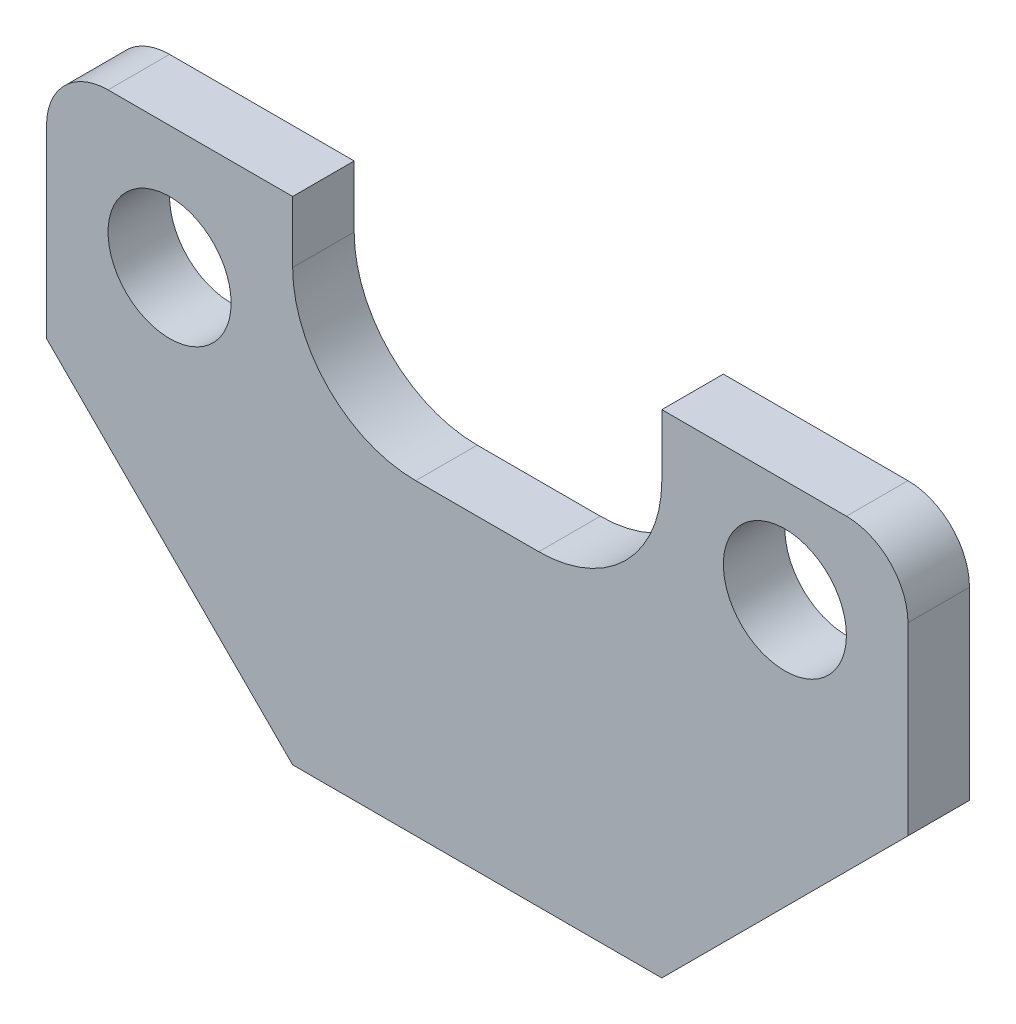
ISO-10303-21;
HEADER;
FILE_DESCRIPTION(('STEP AP214'),'2;1');
FILE_NAME('part.step','',(''),(''),'','','');
FILE_SCHEMA(('AUTOMOTIVE_DESIGN { 1 0 10303 214 1 1 1 1 }'));
ENDSEC;
DATA;
#1=APPLICATION_CONTEXT('core data for automotive mechanical design processes');
#2=APPLICATION_PROTOCOL_DEFINITION('international standard','automotive_design',2000,#1);
#3=PRODUCT_CONTEXT('',#1,'mechanical');
#4=PRODUCT('Part','Part','',(#3));
#5=PRODUCT_RELATED_PRODUCT_CATEGORY('part','',(#4));
#6=PRODUCT_DEFINITION_FORMATION('','',#4);
#7=PRODUCT_DEFINITION_CONTEXT('part definition',#1,'design');
#8=PRODUCT_DEFINITION('design','',#6,#7);
#9=PRODUCT_DEFINITION_SHAPE('','',#8);
#10=(LENGTH_UNIT() NAMED_UNIT(*) SI_UNIT(.MILLI.,.METRE.));
#11=(NAMED_UNIT(*) PLANE_ANGLE_UNIT() SI_UNIT($,.RADIAN.));
#12=(NAMED_UNIT(*) SI_UNIT($,.STERADIAN.) SOLID_ANGLE_UNIT());
#13=UNCERTAINTY_MEASURE_WITH_UNIT(LENGTH_MEASURE(1.E-05),#10,'distance_accuracy_value','');
#14=(GEOMETRIC_REPRESENTATION_CONTEXT(3) GLOBAL_UNCERTAINTY_ASSIGNED_CONTEXT((#13)) GLOBAL_UNIT_ASSIGNED_CONTEXT((#10,
#11,#12)) REPRESENTATION_CONTEXT('',''));
#15=CARTESIAN_POINT('',(0.,0.,0.));
#16=DIRECTION('',(0.,0.,1.));
#17=DIRECTION('',(1.,0.,0.));
#18=AXIS2_PLACEMENT_3D('',#15,#16,#17);
#19=CARTESIAN_POINT('',(0.,0.,5.));
#20=DIRECTION('',(0.707106781186548,0.707106781186548,0.));
#21=DIRECTION('',(-0.707106781186548,0.707106781186548,0.));
#22=AXIS2_PLACEMENT_3D('',#19,#20,#21);
#23=PLANE('',#22);
#24=DIRECTION('',(0.707106781186548,-0.707106781186548,0.));
#25=VECTOR('',#24,1.);
#26=CARTESIAN_POINT('',(0.,0.,0.));
#27=LINE('',#26,#25);
#28=CARTESIAN_POINT('',(-20.,20.,0.));
#29=VERTEX_POINT('',#28);
#30=CARTESIAN_POINT('',(0.,0.,0.));
#31=VERTEX_POINT('',#30);
#32=EDGE_CURVE('E169',#29,#31,#27,.T.);
#33=ORIENTED_EDGE('',*,*,#32,.T.);
#34=DIRECTION('',(0.,0.,-1.));
#35=VECTOR('',#34,1.);
#36=CARTESIAN_POINT('',(0.,0.,5.));
#37=LINE('',#36,#35);
#38=CARTESIAN_POINT('',(0.,0.,5.));
#39=VERTEX_POINT('',#38);
#40=EDGE_CURVE('E147',#39,#31,#37,.T.);
#41=ORIENTED_EDGE('',*,*,#40,.F.);
#42=DIRECTION('',(0.707106781186548,-0.707106781186548,0.));
#43=VECTOR('',#42,1.);
#44=CARTESIAN_POINT('',(0.,0.,5.));
#45=LINE('',#44,#43);
#46=CARTESIAN_POINT('',(-20.,20.,5.));
#47=VERTEX_POINT('',#46);
#48=EDGE_CURVE('E156',#47,#39,#45,.T.);
#49=ORIENTED_EDGE('',*,*,#48,.F.);
#50=DIRECTION('',(0.,0.,-1.));
#51=VECTOR('',#50,1.);
#52=CARTESIAN_POINT('',(-20.,20.,5.));
#53=LINE('',#52,#51);
#54=EDGE_CURVE('E203',#47,#29,#53,.T.);
#55=ORIENTED_EDGE('',*,*,#54,.T.);
#56=EDGE_LOOP('',(#33,#41,#49,#55));
#57=FACE_BOUND('',#56,.T.);
#58=ADVANCED_FACE('F44',(#57),#23,.F.);
#59=CARTESIAN_POINT('',(0.,0.,5.));
#60=DIRECTION('',(0.,1.,0.));
#61=DIRECTION('',(0.,0.,1.));
#62=AXIS2_PLACEMENT_3D('',#59,#60,#61);
#63=PLANE('',#62);
#64=DIRECTION('',(1.,0.,0.));
#65=VECTOR('',#64,1.);
#66=CARTESIAN_POINT('',(0.,0.,0.));
#67=LINE('',#66,#65);
#68=CARTESIAN_POINT('',(30.,0.,0.));
#69=VERTEX_POINT('',#68);
#70=EDGE_CURVE('E240',#31,#69,#67,.T.);
#71=ORIENTED_EDGE('',*,*,#70,.T.);
#72=DIRECTION('',(0.,0.,-1.));
#73=VECTOR('',#72,1.);
#74=CARTESIAN_POINT('',(30.,0.,5.));
#75=LINE('',#74,#73);
#76=CARTESIAN_POINT('',(30.,0.,5.));
#77=VERTEX_POINT('',#76);
#78=EDGE_CURVE('E153',#77,#69,#75,.T.);
#79=ORIENTED_EDGE('',*,*,#78,.F.);
#80=DIRECTION('',(1.,0.,0.));
#81=VECTOR('',#80,1.);
#82=CARTESIAN_POINT('',(0.,0.,5.));
#83=LINE('',#82,#81);
#84=EDGE_CURVE('E148',#39,#77,#83,.T.);
#85=ORIENTED_EDGE('',*,*,#84,.F.);
#86=ORIENTED_EDGE('',*,*,#40,.T.);
#87=EDGE_LOOP('',(#71,#79,#85,#86));
#88=FACE_BOUND('',#87,.T.);
#89=ADVANCED_FACE('F146',(#88),#63,.F.);
#90=CARTESIAN_POINT('',(30.,0.,5.));
#91=DIRECTION('',(-0.707106781186547,0.707106781186548,0.));
#92=DIRECTION('',(-0.707106781186548,-0.707106781186547,0.));
#93=AXIS2_PLACEMENT_3D('',#90,#91,#92);
#94=PLANE('',#93);
#95=DIRECTION('',(0.707106781186548,0.707106781186547,0.));
#96=VECTOR('',#95,1.);
#97=CARTESIAN_POINT('',(30.,0.,0.));
#98=LINE('',#97,#96);
#99=CARTESIAN_POINT('',(50.,20.,0.));
#100=VERTEX_POINT('',#99);
#101=EDGE_CURVE('E234',#69,#100,#98,.T.);
#102=ORIENTED_EDGE('',*,*,#101,.T.);
#103=DIRECTION('',(0.,0.,-1.));
#104=VECTOR('',#103,1.);
#105=CARTESIAN_POINT('',(50.,20.,5.));
#106=LINE('',#105,#104);
#107=CARTESIAN_POINT('',(50.,20.,5.));
#108=VERTEX_POINT('',#107);
#109=EDGE_CURVE('E173',#108,#100,#106,.T.);
#110=ORIENTED_EDGE('',*,*,#109,.F.);
#111=DIRECTION('',(0.707106781186548,0.707106781186547,0.));
#112=VECTOR('',#111,1.);
#113=CARTESIAN_POINT('',(30.,0.,5.));
#114=LINE('',#113,#112);
#115=EDGE_CURVE('E154',#77,#108,#114,.T.);
#116=ORIENTED_EDGE('',*,*,#115,.F.);
#117=ORIENTED_EDGE('',*,*,#78,.T.);
#118=EDGE_LOOP('',(#102,#110,#116,#117));
#119=FACE_BOUND('',#118,.T.);
#120=ADVANCED_FACE('F262',(#119),#94,.F.);
#121=CARTESIAN_POINT('',(50.,40.,5.));
#122=DIRECTION('',(-1.,0.,0.));
#123=DIRECTION('',(0.,0.,1.));
#124=AXIS2_PLACEMENT_3D('',#121,#122,#123);
#125=PLANE('',#124);
#126=DIRECTION('',(0.,1.,0.));
#127=VECTOR('',#126,1.);
#128=CARTESIAN_POINT('',(50.,40.,0.));
#129=LINE('',#128,#127);
#130=CARTESIAN_POINT('',(50.,35.,0.));
#131=VERTEX_POINT('',#130);
#132=EDGE_CURVE('E227',#100,#131,#129,.T.);
#133=ORIENTED_EDGE('',*,*,#132,.T.);
#134=DIRECTION('',(0.,0.,-1.));
#135=VECTOR('',#134,1.);
#136=CARTESIAN_POINT('',(50.,35.,5.));
#137=LINE('',#136,#135);
#138=CARTESIAN_POINT('',(50.,35.,5.));
#139=VERTEX_POINT('',#138);
#140=EDGE_CURVE('E182',#131,#139,#137,.F.);
#141=ORIENTED_EDGE('',*,*,#140,.T.);
#142=DIRECTION('',(0.,1.,0.));
#143=VECTOR('',#142,1.);
#144=CARTESIAN_POINT('',(50.,40.,5.));
#145=LINE('',#144,#143);
#146=EDGE_CURVE('E228',#108,#139,#145,.T.);
#147=ORIENTED_EDGE('',*,*,#146,.F.);
#148=ORIENTED_EDGE('',*,*,#109,.T.);
#149=EDGE_LOOP('',(#133,#141,#147,#148));
#150=FACE_BOUND('',#149,.T.);
#151=ADVANCED_FACE('F226',(#150),#125,.F.);
#152=CARTESIAN_POINT('',(30.,40.,5.));
#153=DIRECTION('',(0.,-1.,0.));
#154=DIRECTION('',(0.,0.,-1.));
#155=AXIS2_PLACEMENT_3D('',#152,#153,#154);
#156=PLANE('',#155);
#157=DIRECTION('',(-1.,0.,0.));
#158=VECTOR('',#157,1.);
#159=CARTESIAN_POINT('',(30.,40.,5.));
#160=LINE('',#159,#158);
#161=CARTESIAN_POINT('',(45.,40.,5.));
#162=VERTEX_POINT('',#161);
#163=CARTESIAN_POINT('',(30.,40.,5.));
#164=VERTEX_POINT('',#163);
#165=EDGE_CURVE('E266',#162,#164,#160,.T.);
#166=ORIENTED_EDGE('',*,*,#165,.F.);
#167=DIRECTION('',(0.,0.,-1.));
#168=VECTOR('',#167,1.);
#169=CARTESIAN_POINT('',(45.,40.,5.));
#170=LINE('',#169,#168);
#171=CARTESIAN_POINT('',(45.,40.,0.));
#172=VERTEX_POINT('',#171);
#173=EDGE_CURVE('E166',#162,#172,#170,.T.);
#174=ORIENTED_EDGE('',*,*,#173,.T.);
#175=DIRECTION('',(-1.,0.,0.));
#176=VECTOR('',#175,1.);
#177=CARTESIAN_POINT('',(30.,40.,0.));
#178=LINE('',#177,#176);
#179=CARTESIAN_POINT('',(30.,40.,0.));
#180=VERTEX_POINT('',#179);
#181=EDGE_CURVE('E232',#172,#180,#178,.T.);
#182=ORIENTED_EDGE('',*,*,#181,.T.);
#183=DIRECTION('',(0.,0.,-1.));
#184=VECTOR('',#183,1.);
#185=CARTESIAN_POINT('',(30.,40.,5.));
#186=LINE('',#185,#184);
#187=EDGE_CURVE('E217',#164,#180,#186,.T.);
#188=ORIENTED_EDGE('',*,*,#187,.F.);
#189=EDGE_LOOP('',(#166,#174,#182,#188));
#190=FACE_BOUND('',#189,.T.);
#191=ADVANCED_FACE('F296',(#190),#156,.F.);
#192=CARTESIAN_POINT('',(30.,35.,5.));
#193=DIRECTION('',(1.,0.,0.));
#194=DIRECTION('',(0.,0.,-1.));
#195=AXIS2_PLACEMENT_3D('',#192,#193,#194);
#196=PLANE('',#195);
#197=DIRECTION('',(0.,-1.,0.));
#198=VECTOR('',#197,1.);
#199=CARTESIAN_POINT('',(30.,35.,0.));
#200=LINE('',#199,#198);
#201=CARTESIAN_POINT('',(30.,35.,0.));
#202=VERTEX_POINT('',#201);
#203=EDGE_CURVE('E231',#180,#202,#200,.T.);
#204=ORIENTED_EDGE('',*,*,#203,.T.);
#205=DIRECTION('',(0.,0.,-1.));
#206=VECTOR('',#205,1.);
#207=CARTESIAN_POINT('',(30.,35.,5.));
#208=LINE('',#207,#206);
#209=CARTESIAN_POINT('',(30.,35.,5.));
#210=VERTEX_POINT('',#209);
#211=EDGE_CURVE('E214',#210,#202,#208,.T.);
#212=ORIENTED_EDGE('',*,*,#211,.F.);
#213=DIRECTION('',(0.,-1.,0.));
#214=VECTOR('',#213,1.);
#215=CARTESIAN_POINT('',(30.,35.,5.));
#216=LINE('',#215,#214);
#217=EDGE_CURVE('E269',#164,#210,#216,.T.);
#218=ORIENTED_EDGE('',*,*,#217,.F.);
#219=ORIENTED_EDGE('',*,*,#187,.T.);
#220=EDGE_LOOP('',(#204,#212,#218,#219));
#221=FACE_BOUND('',#220,.T.);
#222=ADVANCED_FACE('F295',(#221),#196,.F.);
#223=CARTESIAN_POINT('',(20.,35.,5.));
#224=DIRECTION('',(0.,0.,-1.));
#225=DIRECTION('',(-1.,0.,0.));
#226=AXIS2_PLACEMENT_3D('',#223,#224,#225);
#227=CYLINDRICAL_SURFACE('',#226,10.);
#228=CARTESIAN_POINT('',(20.,35.,0.));
#229=DIRECTION('',(0.,0.,-1.));
#230=DIRECTION('',(1.,0.,0.));
#231=AXIS2_PLACEMENT_3D('',#228,#229,#230);
#232=CIRCLE('',#231,10.);
#233=CARTESIAN_POINT('',(20.,25.,0.));
#234=VERTEX_POINT('',#233);
#235=EDGE_CURVE('E242',#202,#234,#232,.T.);
#236=ORIENTED_EDGE('',*,*,#235,.T.);
#237=DIRECTION('',(0.,0.,-1.));
#238=VECTOR('',#237,1.);
#239=CARTESIAN_POINT('',(20.,25.,5.));
#240=LINE('',#239,#238);
#241=CARTESIAN_POINT('',(20.,25.,5.));
#242=VERTEX_POINT('',#241);
#243=EDGE_CURVE('E215',#242,#234,#240,.T.);
#244=ORIENTED_EDGE('',*,*,#243,.F.);
#245=CARTESIAN_POINT('',(20.,35.,5.));
#246=DIRECTION('',(0.,0.,-1.));
#247=DIRECTION('',(1.,0.,0.));
#248=AXIS2_PLACEMENT_3D('',#245,#246,#247);
#249=CIRCLE('',#248,10.);
#250=EDGE_CURVE('E275',#210,#242,#249,.T.);
#251=ORIENTED_EDGE('',*,*,#250,.F.);
#252=ORIENTED_EDGE('',*,*,#211,.T.);
#253=EDGE_LOOP('',(#236,#244,#251,#252));
#254=FACE_BOUND('',#253,.T.);
#255=ADVANCED_FACE('F287',(#254),#227,.F.);
#256=CARTESIAN_POINT('',(10.,25.,5.));
#257=DIRECTION('',(0.,-1.,0.));
#258=DIRECTION('',(0.,0.,-1.));
#259=AXIS2_PLACEMENT_3D('',#256,#257,#258);
#260=PLANE('',#259);
#261=DIRECTION('',(-1.,0.,0.));
#262=VECTOR('',#261,1.);
#263=CARTESIAN_POINT('',(10.,25.,0.));
#264=LINE('',#263,#262);
#265=CARTESIAN_POINT('',(10.,25.,0.));
#266=VERTEX_POINT('',#265);
#267=EDGE_CURVE('E243',#234,#266,#264,.T.);
#268=ORIENTED_EDGE('',*,*,#267,.T.);
#269=DIRECTION('',(0.,0.,-1.));
#270=VECTOR('',#269,1.);
#271=CARTESIAN_POINT('',(10.,25.,5.));
#272=LINE('',#271,#270);
#273=CARTESIAN_POINT('',(10.,25.,5.));
#274=VERTEX_POINT('',#273);
#275=EDGE_CURVE('E207',#274,#266,#272,.T.);
#276=ORIENTED_EDGE('',*,*,#275,.F.);
#277=DIRECTION('',(-1.,0.,0.));
#278=VECTOR('',#277,1.);
#279=CARTESIAN_POINT('',(10.,25.,5.));
#280=LINE('',#279,#278);
#281=EDGE_CURVE('E273',#242,#274,#280,.T.);
#282=ORIENTED_EDGE('',*,*,#281,.F.);
#283=ORIENTED_EDGE('',*,*,#243,.T.);
#284=EDGE_LOOP('',(#268,#276,#282,#283));
#285=FACE_BOUND('',#284,.T.);
#286=ADVANCED_FACE('F283',(#285),#260,.F.);
#287=CARTESIAN_POINT('',(10.,35.,5.));
#288=DIRECTION('',(0.,0.,-1.));
#289=DIRECTION('',(-1.,0.,0.));
#290=AXIS2_PLACEMENT_3D('',#287,#288,#289);
#291=CYLINDRICAL_SURFACE('',#290,10.);
#292=CARTESIAN_POINT('',(10.,35.,0.));
#293=DIRECTION('',(0.,0.,-1.));
#294=DIRECTION('',(1.,0.,0.));
#295=AXIS2_PLACEMENT_3D('',#292,#293,#294);
#296=CIRCLE('',#295,10.);
#297=CARTESIAN_POINT('',(0.,35.,0.));
#298=VERTEX_POINT('',#297);
#299=EDGE_CURVE('E248',#266,#298,#296,.T.);
#300=ORIENTED_EDGE('',*,*,#299,.T.);
#301=DIRECTION('',(0.,0.,-1.));
#302=VECTOR('',#301,1.);
#303=CARTESIAN_POINT('',(0.,35.,5.));
#304=LINE('',#303,#302);
#305=CARTESIAN_POINT('',(0.,35.,5.));
#306=VERTEX_POINT('',#305);
#307=EDGE_CURVE('E206',#306,#298,#304,.T.);
#308=ORIENTED_EDGE('',*,*,#307,.F.);
#309=CARTESIAN_POINT('',(10.,35.,5.));
#310=DIRECTION('',(0.,0.,-1.));
#311=DIRECTION('',(1.,0.,0.));
#312=AXIS2_PLACEMENT_3D('',#309,#310,#311);
#313=CIRCLE('',#312,10.);
#314=EDGE_CURVE('E259',#274,#306,#313,.T.);
#315=ORIENTED_EDGE('',*,*,#314,.F.);
#316=ORIENTED_EDGE('',*,*,#275,.T.);
#317=EDGE_LOOP('',(#300,#308,#315,#316));
#318=FACE_BOUND('',#317,.T.);
#319=ADVANCED_FACE('F276',(#318),#291,.F.);
#320=CARTESIAN_POINT('',(0.,40.,5.));
#321=DIRECTION('',(-1.,0.,0.));
#322=DIRECTION('',(0.,0.,1.));
#323=AXIS2_PLACEMENT_3D('',#320,#321,#322);
#324=PLANE('',#323);
#325=DIRECTION('',(0.,1.,0.));
#326=VECTOR('',#325,1.);
#327=CARTESIAN_POINT('',(0.,40.,0.));
#328=LINE('',#327,#326);
#329=CARTESIAN_POINT('',(0.,40.,0.));
#330=VERTEX_POINT('',#329);
#331=EDGE_CURVE('E197',#298,#330,#328,.T.);
#332=ORIENTED_EDGE('',*,*,#331,.T.);
#333=DIRECTION('',(0.,0.,-1.));
#334=VECTOR('',#333,1.);
#335=CARTESIAN_POINT('',(0.,40.,5.));
#336=LINE('',#335,#334);
#337=CARTESIAN_POINT('',(0.,40.,5.));
#338=VERTEX_POINT('',#337);
#339=EDGE_CURVE('E201',#338,#330,#336,.T.);
#340=ORIENTED_EDGE('',*,*,#339,.F.);
#341=DIRECTION('',(0.,1.,0.));
#342=VECTOR('',#341,1.);
#343=CARTESIAN_POINT('',(0.,40.,5.));
#344=LINE('',#343,#342);
#345=EDGE_CURVE('E258',#306,#338,#344,.T.);
#346=ORIENTED_EDGE('',*,*,#345,.F.);
#347=ORIENTED_EDGE('',*,*,#307,.T.);
#348=EDGE_LOOP('',(#332,#340,#346,#347));
#349=FACE_BOUND('',#348,.T.);
#350=ADVANCED_FACE('F246',(#349),#324,.F.);
#351=CARTESIAN_POINT('',(0.,40.,5.));
#352=DIRECTION('',(0.,-1.,0.));
#353=DIRECTION('',(0.,0.,-1.));
#354=AXIS2_PLACEMENT_3D('',#351,#352,#353);
#355=PLANE('',#354);
#356=DIRECTION('',(-1.,0.,0.));
#357=VECTOR('',#356,1.);
#358=CARTESIAN_POINT('',(0.,40.,0.));
#359=LINE('',#358,#357);
#360=CARTESIAN_POINT('',(-15.,40.,0.));
#361=VERTEX_POINT('',#360);
#362=EDGE_CURVE('E191',#330,#361,#359,.T.);
#363=ORIENTED_EDGE('',*,*,#362,.T.);
#364=DIRECTION('',(0.,0.,-1.));
#365=VECTOR('',#364,1.);
#366=CARTESIAN_POINT('',(-15.,40.,5.));
#367=LINE('',#366,#365);
#368=CARTESIAN_POINT('',(-15.,40.,5.));
#369=VERTEX_POINT('',#368);
#370=EDGE_CURVE('E11',#361,#369,#367,.F.);
#371=ORIENTED_EDGE('',*,*,#370,.T.);
#372=DIRECTION('',(-1.,0.,0.));
#373=VECTOR('',#372,1.);
#374=CARTESIAN_POINT('',(0.,40.,5.));
#375=LINE('',#374,#373);
#376=EDGE_CURVE('E254',#338,#369,#375,.T.);
#377=ORIENTED_EDGE('',*,*,#376,.F.);
#378=ORIENTED_EDGE('',*,*,#339,.T.);
#379=EDGE_LOOP('',(#363,#371,#377,#378));
#380=FACE_BOUND('',#379,.T.);
#381=ADVANCED_FACE('F255',(#380),#355,.F.);
#382=CARTESIAN_POINT('',(-20.,40.,5.));
#383=DIRECTION('',(1.,0.,0.));
#384=DIRECTION('',(0.,0.,-1.));
#385=AXIS2_PLACEMENT_3D('',#382,#383,#384);
#386=PLANE('',#385);
#387=DIRECTION('',(0.,-1.,0.));
#388=VECTOR('',#387,1.);
#389=CARTESIAN_POINT('',(-20.,40.,5.));
#390=LINE('',#389,#388);
#391=CARTESIAN_POINT('',(-20.,35.,5.));
#392=VERTEX_POINT('',#391);
#393=EDGE_CURVE('E161',#392,#47,#390,.T.);
#394=ORIENTED_EDGE('',*,*,#393,.F.);
#395=DIRECTION('',(0.,0.,-1.));
#396=VECTOR('',#395,1.);
#397=CARTESIAN_POINT('',(-20.,35.,5.));
#398=LINE('',#397,#396);
#399=CARTESIAN_POINT('',(-20.,35.,0.));
#400=VERTEX_POINT('',#399);
#401=EDGE_CURVE('E52',#392,#400,#398,.T.);
#402=ORIENTED_EDGE('',*,*,#401,.T.);
#403=DIRECTION('',(0.,-1.,0.));
#404=VECTOR('',#403,1.);
#405=CARTESIAN_POINT('',(-20.,40.,0.));
#406=LINE('',#405,#404);
#407=EDGE_CURVE('E164',#400,#29,#406,.T.);
#408=ORIENTED_EDGE('',*,*,#407,.T.);
#409=ORIENTED_EDGE('',*,*,#54,.F.);
#410=EDGE_LOOP('',(#394,#402,#408,#409));
#411=FACE_BOUND('',#410,.T.);
#412=ADVANCED_FACE('F188',(#411),#386,.F.);
#413=CARTESIAN_POINT('',(10.,35.,5.));
#414=DIRECTION('',(0.,0.,1.));
#415=DIRECTION('',(1.,0.,0.));
#416=AXIS2_PLACEMENT_3D('',#413,#414,#415);
#417=PLANE('',#416);
#418=CARTESIAN_POINT('',(40.,31.6094695208061,5.));
#419=DIRECTION('',(0.,0.,1.));
#420=DIRECTION('',(1.,0.,0.));
#421=AXIS2_PLACEMENT_3D('',#418,#419,#420);
#422=CIRCLE('',#421,5.);
#423=CARTESIAN_POINT('',(45.,31.6094695208061,5.));
#424=VERTEX_POINT('',#423);
#425=EDGE_CURVE('E357',#424,#424,#422,.T.);
#426=ORIENTED_EDGE('',*,*,#425,.F.);
#427=EDGE_LOOP('',(#426));
#428=FACE_BOUND('',#427,.T.);
#429=CARTESIAN_POINT('',(-10.,30.,5.));
#430=DIRECTION('',(0.,0.,1.));
#431=DIRECTION('',(1.,0.,0.));
#432=AXIS2_PLACEMENT_3D('',#429,#430,#431);
#433=CIRCLE('',#432,5.);
#434=CARTESIAN_POINT('',(-5.,30.,5.));
#435=VERTEX_POINT('',#434);
#436=EDGE_CURVE('E352',#435,#435,#433,.T.);
#437=ORIENTED_EDGE('',*,*,#436,.F.);
#438=EDGE_LOOP('',(#437));
#439=FACE_BOUND('',#438,.T.);
#440=ORIENTED_EDGE('',*,*,#146,.T.);
#441=CARTESIAN_POINT('',(45.,35.,5.));
#442=DIRECTION('',(0.,0.,1.));
#443=DIRECTION('',(1.,0.,0.));
#444=AXIS2_PLACEMENT_3D('',#441,#442,#443);
#445=CIRCLE('',#444,5.);
#446=EDGE_CURVE('E184',#139,#162,#445,.T.);
#447=ORIENTED_EDGE('',*,*,#446,.T.);
#448=ORIENTED_EDGE('',*,*,#165,.T.);
#449=ORIENTED_EDGE('',*,*,#217,.T.);
#450=ORIENTED_EDGE('',*,*,#250,.T.);
#451=ORIENTED_EDGE('',*,*,#281,.T.);
#452=ORIENTED_EDGE('',*,*,#314,.T.);
#453=ORIENTED_EDGE('',*,*,#345,.T.);
#454=ORIENTED_EDGE('',*,*,#376,.T.);
#455=CARTESIAN_POINT('',(-15.,35.,5.));
#456=DIRECTION('',(0.,0.,1.));
#457=DIRECTION('',(1.,0.,0.));
#458=AXIS2_PLACEMENT_3D('',#455,#456,#457);
#459=CIRCLE('',#458,5.);
#460=EDGE_CURVE('E58',#369,#392,#459,.T.);
#461=ORIENTED_EDGE('',*,*,#460,.T.);
#462=ORIENTED_EDGE('',*,*,#393,.T.);
#463=ORIENTED_EDGE('',*,*,#48,.T.);
#464=ORIENTED_EDGE('',*,*,#84,.T.);
#465=ORIENTED_EDGE('',*,*,#115,.T.);
#466=EDGE_LOOP('',(#440,#447,#448,#449,#450,#451,#452,#453,#454,#461,#462,#463,#464,#465));
#467=FACE_BOUND('',#466,.T.);
#468=ADVANCED_FACE('F159',(#428,#439,#467),#417,.T.);
#469=CARTESIAN_POINT('',(10.,35.,0.));
#470=DIRECTION('',(0.,0.,1.));
#471=DIRECTION('',(1.,0.,0.));
#472=AXIS2_PLACEMENT_3D('',#469,#470,#471);
#473=PLANE('',#472);
#474=CARTESIAN_POINT('',(40.,31.6094695208061,0.));
#475=DIRECTION('',(0.,0.,1.));
#476=DIRECTION('',(1.,0.,0.));
#477=AXIS2_PLACEMENT_3D('',#474,#475,#476);
#478=CIRCLE('',#477,5.);
#479=CARTESIAN_POINT('',(45.,31.6094695208061,0.));
#480=VERTEX_POINT('',#479);
#481=EDGE_CURVE('E353',#480,#480,#478,.T.);
#482=ORIENTED_EDGE('',*,*,#481,.T.);
#483=EDGE_LOOP('',(#482));
#484=FACE_BOUND('',#483,.T.);
#485=CARTESIAN_POINT('',(-10.,30.,0.));
#486=DIRECTION('',(0.,0.,1.));
#487=DIRECTION('',(1.,0.,0.));
#488=AXIS2_PLACEMENT_3D('',#485,#486,#487);
#489=CIRCLE('',#488,5.);
#490=CARTESIAN_POINT('',(-5.,30.,0.));
#491=VERTEX_POINT('',#490);
#492=EDGE_CURVE('E263',#491,#491,#489,.T.);
#493=ORIENTED_EDGE('',*,*,#492,.T.);
#494=EDGE_LOOP('',(#493));
#495=FACE_BOUND('',#494,.T.);
#496=ORIENTED_EDGE('',*,*,#181,.F.);
#497=CARTESIAN_POINT('',(45.,35.,0.));
#498=DIRECTION('',(0.,0.,1.));
#499=DIRECTION('',(1.,0.,0.));
#500=AXIS2_PLACEMENT_3D('',#497,#498,#499);
#501=CIRCLE('',#500,5.);
#502=EDGE_CURVE('E180',#172,#131,#501,.F.);
#503=ORIENTED_EDGE('',*,*,#502,.T.);
#504=ORIENTED_EDGE('',*,*,#132,.F.);
#505=ORIENTED_EDGE('',*,*,#101,.F.);
#506=ORIENTED_EDGE('',*,*,#70,.F.);
#507=ORIENTED_EDGE('',*,*,#32,.F.);
#508=ORIENTED_EDGE('',*,*,#407,.F.);
#509=CARTESIAN_POINT('',(-15.,35.,0.));
#510=DIRECTION('',(0.,0.,1.));
#511=DIRECTION('',(1.,0.,0.));
#512=AXIS2_PLACEMENT_3D('',#509,#510,#511);
#513=CIRCLE('',#512,5.);
#514=EDGE_CURVE('E172',#400,#361,#513,.F.);
#515=ORIENTED_EDGE('',*,*,#514,.T.);
#516=ORIENTED_EDGE('',*,*,#362,.F.);
#517=ORIENTED_EDGE('',*,*,#331,.F.);
#518=ORIENTED_EDGE('',*,*,#299,.F.);
#519=ORIENTED_EDGE('',*,*,#267,.F.);
#520=ORIENTED_EDGE('',*,*,#235,.F.);
#521=ORIENTED_EDGE('',*,*,#203,.F.);
#522=EDGE_LOOP('',(#496,#503,#504,#505,#506,#507,#508,#515,#516,#517,#518,#519,#520,#521));
#523=FACE_BOUND('',#522,.T.);
#524=ADVANCED_FACE('F192',(#484,#495,#523),#473,.F.);
#525=CARTESIAN_POINT('',(-10.,30.,0.));
#526=DIRECTION('',(0.,0.,1.));
#527=DIRECTION('',(1.,0.,0.));
#528=AXIS2_PLACEMENT_3D('',#525,#526,#527);
#529=CYLINDRICAL_SURFACE('',#528,5.);
#530=ORIENTED_EDGE('',*,*,#492,.F.);
#531=EDGE_LOOP('',(#530));
#532=FACE_BOUND('',#531,.T.);
#533=ORIENTED_EDGE('',*,*,#436,.T.);
#534=EDGE_LOOP('',(#533));
#535=FACE_BOUND('',#534,.T.);
#536=ADVANCED_FACE('F307',(#532,#535),#529,.F.);
#537=CARTESIAN_POINT('',(40.,31.6094695208061,0.));
#538=DIRECTION('',(0.,0.,1.));
#539=DIRECTION('',(1.,0.,0.));
#540=AXIS2_PLACEMENT_3D('',#537,#538,#539);
#541=CYLINDRICAL_SURFACE('',#540,5.);
#542=ORIENTED_EDGE('',*,*,#481,.F.);
#543=EDGE_LOOP('',(#542));
#544=FACE_BOUND('',#543,.T.);
#545=ORIENTED_EDGE('',*,*,#425,.T.);
#546=EDGE_LOOP('',(#545));
#547=FACE_BOUND('',#546,.T.);
#548=ADVANCED_FACE('F304',(#544,#547),#541,.F.);
#549=CARTESIAN_POINT('',(45.,35.,5.));
#550=DIRECTION('',(0.,0.,-1.));
#551=DIRECTION('',(-1.,0.,0.));
#552=AXIS2_PLACEMENT_3D('',#549,#550,#551);
#553=CYLINDRICAL_SURFACE('',#552,5.);
#554=ORIENTED_EDGE('',*,*,#446,.F.);
#555=ORIENTED_EDGE('',*,*,#140,.F.);
#556=ORIENTED_EDGE('',*,*,#502,.F.);
#557=ORIENTED_EDGE('',*,*,#173,.F.);
#558=EDGE_LOOP('',(#554,#555,#556,#557));
#559=FACE_BOUND('',#558,.T.);
#560=ADVANCED_FACE('F300',(#559),#553,.T.);
#561=CARTESIAN_POINT('',(-15.,35.,5.));
#562=DIRECTION('',(0.,0.,-1.));
#563=DIRECTION('',(-1.,0.,0.));
#564=AXIS2_PLACEMENT_3D('',#561,#562,#563);
#565=CYLINDRICAL_SURFACE('',#564,5.);
#566=ORIENTED_EDGE('',*,*,#460,.F.);
#567=ORIENTED_EDGE('',*,*,#370,.F.);
#568=ORIENTED_EDGE('',*,*,#514,.F.);
#569=ORIENTED_EDGE('',*,*,#401,.F.);
#570=EDGE_LOOP('',(#566,#567,#568,#569));
#571=FACE_BOUND('',#570,.T.);
#572=ADVANCED_FACE('F50',(#571),#565,.T.);
#573=CLOSED_SHELL('',(#58,#89,#120,#151,#191,#222,#255,#286,#319,#350,#381,#412,#468,#524,#536,
#548,#560,#572));
#574=MANIFOLD_SOLID_BREP('B2',#573);
#575=ADVANCED_BREP_SHAPE_REPRESENTATION('',(#18,#574),#14);
#576=SHAPE_DEFINITION_REPRESENTATION(#9,#575);
ENDSEC;
END-ISO-10303-21;
